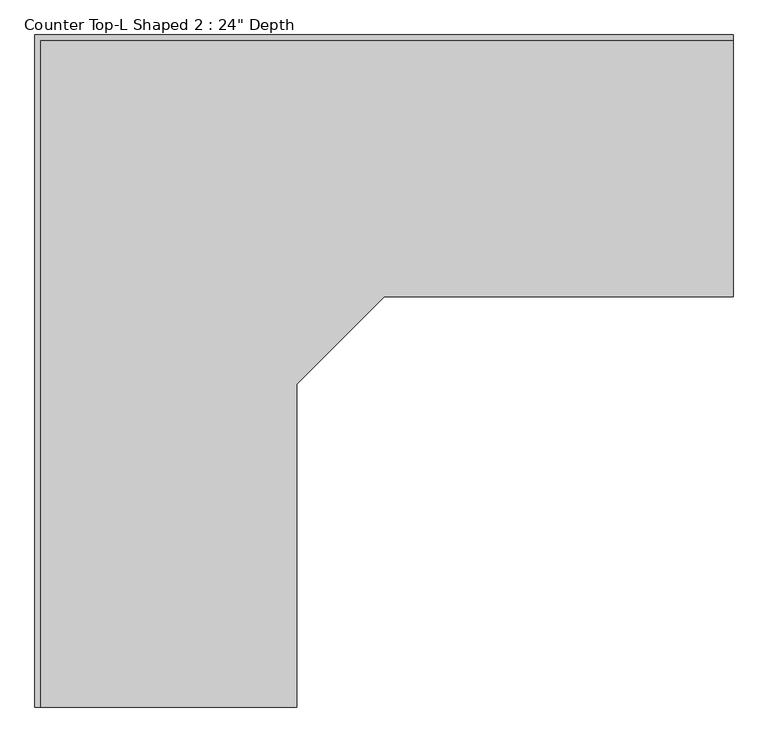
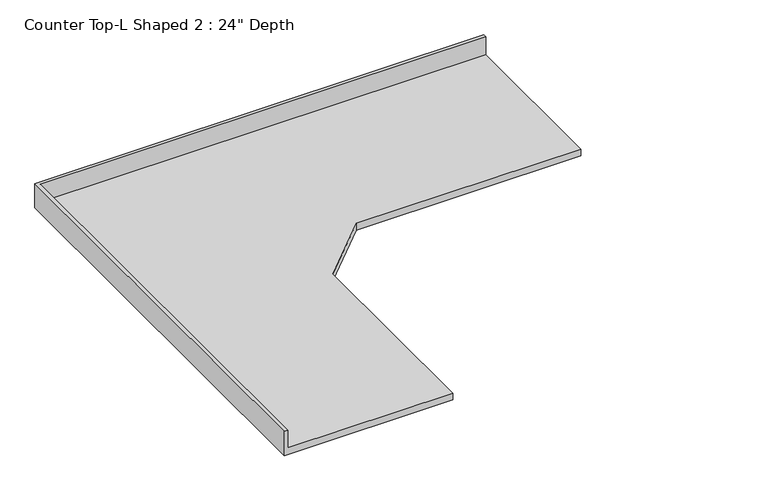
"""IFC4 building model written with IfcOpenShell, lengths in millimetres: furniture geometry."""

from ifc_helpers import new_model, si_unit, origin, place, context, project, spatial, faceted_brep, source, transform, mapped, element, save


def furniture_c973ddc6(model_context):
    return source(origin(), model_context, "Body", "Brep", [
        faceted_brep([(-286.0622951, -2347.331658, 914.4), (-286.0622951, -1219.2, 914.4), (18.7377049, -914.4, 914.4), (1237.9377049, -914.4, 914.4), (1237.9377049, -19.05, 914.4), (-1181.4122951, -19.05, 914.4), (-1181.4122951, -2347.331658, 914.4), (1237.9377049, 0.0, 876.3), (1237.9377049, -914.4, 876.3), (18.7377049, -914.4, 876.3), (-286.0622951, -1219.2, 876.3), (-286.0622951, -2347.331658, 876.3), (-1200.4622951, -2347.331658, 876.3), (-1200.4622951, 0.0, 876.3), (-1200.4622951, 0.0, 1016.0), (1237.9377049, 0.0, 1016.0), (-1200.4622951, -2347.331658, 1016.0), (-1181.4122951, -2347.331658, 1016.0), (1237.9377049, -19.05, 1016.0), (-1181.4122951, -19.05, 1016.0)], [[[0, 1, 2, 3, 4, 5, 6]], [[7, 8, 9, 10, 11, 12, 13]], [[7, 13, 14, 15]], [[13, 12, 16, 14]], [[16, 12, 11, 0, 6, 17]], [[1, 0, 11, 10]], [[2, 1, 10, 9]], [[3, 2, 9, 8]], [[8, 7, 15, 18, 4, 3]], [[14, 16, 17, 19, 18, 15]], [[4, 18, 19, 5]], [[19, 17, 6, 5]]]),
    ])


if __name__ == "__main__":
    model = new_model("IFC4")
    model_context = context("Model", 3, world=origin())
    ifc_project = project(units=[si_unit("LENGTHUNIT", "METRE", prefix="MILLI")], contexts=[model_context])
    site = spatial("IfcSite", under=ifc_project)
    building = spatial("IfcBuilding", under=site)
    placement = place(None, origin())
    furniture_shape = furniture_c973ddc6(model_context)
    element("IfcFurniture", 1, ObjectType="Counter Top-L Shaped 2 : 24\" Depth", at=placement, inside=building, context=model_context, shape_type="MappedRepresentation", body=[
        mapped(furniture_shape, transform((0.0, 0.0, 0.0), x_axis=(1.0, 0.0, 0.0), y_axis=(0.0, 1.0, 0.0), z_axis=(0.0, 0.0, 1.0))),
    ])
    save(model, "model.ifc")

# Revit data of these elements
# Type "Counter Top-L Shaped 2 : 24\" Depth"
#   Assembly Code = "C1030400"
#   Counter Thickness = 0' - 1 1/2"
#   Depth = 3' - 0"
#   Height = 3' - 0"
#   Length - Leg 1 [instance default] = 8' - 0"
#   Length - Leg 2 [instance default] = 6' - 0"
#   Counter Top Material = none
#   Default Elevation = 0
# Element 1 (IfcFurniture, "Counter Top-L Shaped 2 : 24\" Depth")
#   Length - Leg 2 = 7' - 8.41463"
#   Materials on its faces: "Counter Top"
# Materials
#   "Counter Top": class "Wood", colour RGB 226 177 128, transparency 0
